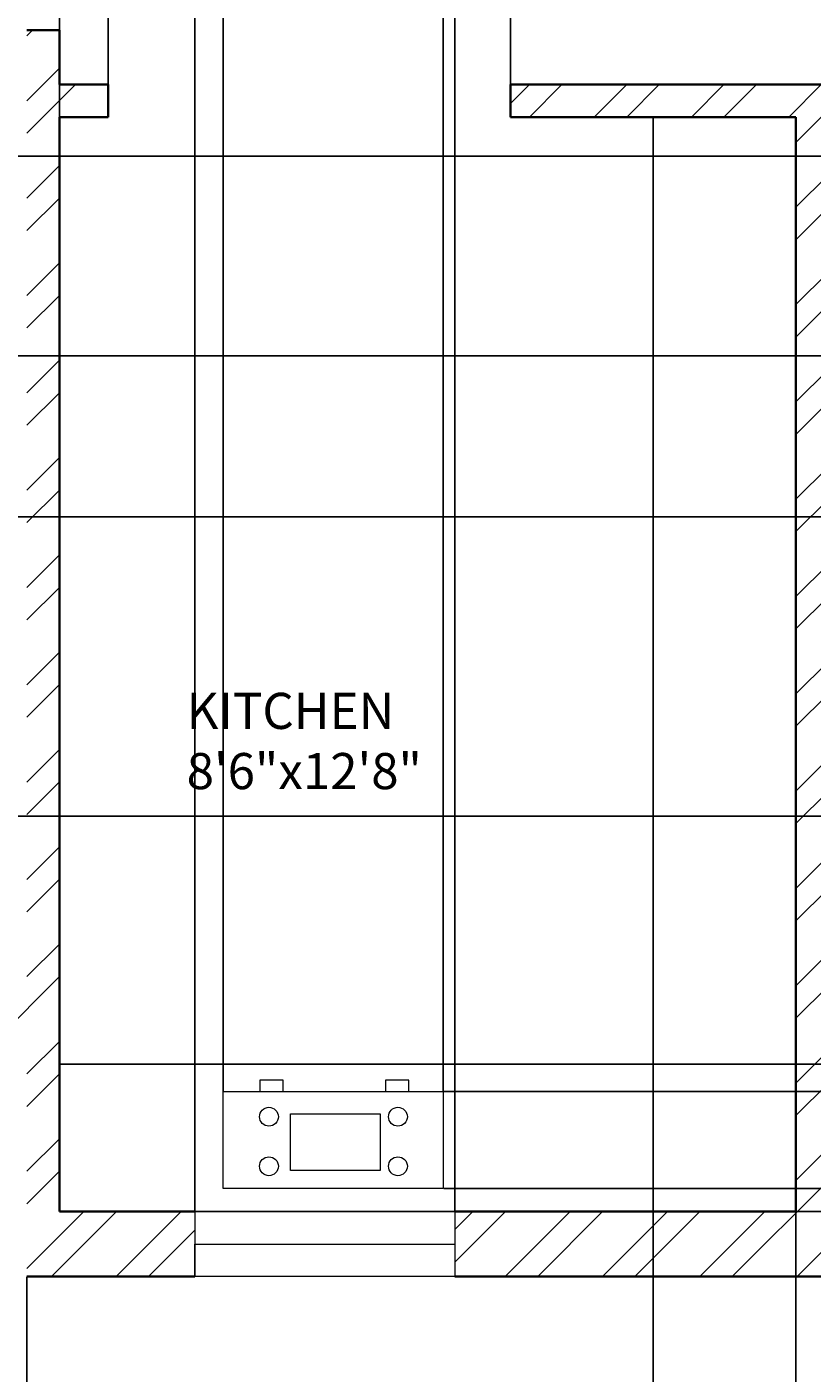
# Model space of a CAD drawing. Units: inches. Extents: x 2529 to 3014, y 1203 to 2262.
# Tile 5 of 13: x 2733 to 2842, y 1560 to 1746. Entities that reach past the tile are written whole.
import ezdxf

# ---------------------------------------------------------------- set-up
doc = ezdxf.new("R2010")
doc.units = ezdxf.units.IN
for name, color, linetype, lineweight in [('A-ANNO-DIMS', 2, 'Continuous', 18), ('A-AREA-IDEN', 7, 'Continuous', 18), ('A-EQPM', 8, 'Continuous', 18), ('A-FLOR-CASE', 7, 'Continuous', 25), ('A-GLAZ', 191, 'Continuous', 18), ('A-WALL', 7, 'Continuous', 35), ('A-WALL-PATT', 143, 'Continuous', 13)]:
    doc.layers.add(name, color=color, linetype=linetype, lineweight=lineweight)
doc.styles.get("Standard").update_dxf_attribs({"font": 'arial.ttf'})
doc.dimstyles.get("Standard").update_dxf_attribs({"dimtxt": 0.18, "dimasz": 0.18, "dimexe": 0.18, "dimexo": 0.0625, "dimgap": 0.09, "dimtad": 0, "dimtih": 1, "dimtoh": 1, "dimdec": 4, "dimzin": 0, "dimdsep": 46, "dimtxsty": 'Standard', "dimcen": 0.09, "dimadec": 0, "dimazin": 0, "dimtfac": 1, "dimtdec": 4, "dimtofl": 0, "dimtmove": 0, "dimatfit": 3, "dimfxl": 1, "dimtolj": 1, "dimtzin": 0, "dimarcsym": 0})

# ---------------------------------------------------------------- blocks, each defined once
blk = doc.blocks.new('*D19')
at = {"layer": 'A-ANNO-DIMS', "color": 0, "lineweight": -2, "transparency": 16777216}
for p, q in [((2839.56, 1582.44), (2839.56, 1483.77)), ((2733.06, 1573.44), (2733.06, 1483.77)), ((2733.24, 1483.95), (2785.92, 1483.95)), ((2839.38, 1483.95), (2786.69, 1483.95))]:
    blk.add_line(p, q, dxfattribs=at)
at = {"layer": 'A-ANNO-DIMS', "color": 0, "transparency": 16777216}
for points in [[(2733.24, 1483.98), (2733.24, 1483.92), (2733.06, 1483.95)], [(2839.38, 1483.98), (2839.38, 1483.92), (2839.56, 1483.95)]]:
    blk.add_solid(points, dxfattribs=at)
at = {"layer": 'Defpoints', "color": 0, "transparency": 16777216}
for p in [(2839.56, 1582.5), (2733.06, 1573.5), (2839.56, 1483.95)]:
    blk.add_point(p, dxfattribs=at)
at = {"layer": 'A-ANNO-DIMS', "color": 0, "transparency": 16777216, "insert": (2786.31, 1483.95), "char_height": 0.18, "attachment_point": 5}
blk.add_mtext('\\A1;106.5', dxfattribs=at)
blk = doc.blocks.new('*D20')
at = {"layer": 'A-ANNO-DIMS', "color": 0, "lineweight": -2, "transparency": 16777216}
for p, q in [((2839.56, 1582.44), (2839.56, 1483.77)), ((2972.06, 1573.44), (2972.06, 1483.77)), ((2839.74, 1483.95), (2905.42, 1483.95)), ((2971.88, 1483.95), (2906.19, 1483.95))]:
    blk.add_line(p, q, dxfattribs=at)
at = {"layer": 'A-ANNO-DIMS', "color": 0, "transparency": 16777216}
for points in [[(2839.74, 1483.98), (2839.74, 1483.92), (2839.56, 1483.95)], [(2971.88, 1483.98), (2971.88, 1483.92), (2972.06, 1483.95)]]:
    blk.add_solid(points, dxfattribs=at)
at = {"layer": 'Defpoints', "color": 0, "transparency": 16777216}
for p in [(2839.56, 1582.5), (2972.06, 1573.5), (2972.06, 1483.95)]:
    blk.add_point(p, dxfattribs=at)
at = {"layer": 'A-ANNO-DIMS', "color": 0, "transparency": 16777216, "insert": (2905.81, 1483.95), "char_height": 0.18, "attachment_point": 5}
blk.add_mtext('\\A1;132.5', dxfattribs=at)
blk = doc.blocks.new('*D36')
at = {"layer": 'A-ANNO-DIMS', "color": 0, "lineweight": -2, "transparency": 16777216}
for p, q in [((2737.56, 1582.57), (2737.56, 2243.11)), ((2737.74, 2242.93), (2746.49, 2242.93)), ((2756.15, 2242.93), (2747.4, 2242.93)), ((2756.33, 1582.57), (2756.33, 2243.11))]:
    blk.add_line(p, q, dxfattribs=at)
at = {"layer": 'A-ANNO-DIMS', "color": 0, "transparency": 16777216}
for points in [[(2737.74, 2242.96), (2737.74, 2242.9), (2737.56, 2242.93)], [(2756.15, 2242.96), (2756.15, 2242.9), (2756.33, 2242.93)]]:
    blk.add_solid(points, dxfattribs=at)
at = {"layer": 'Defpoints', "color": 0, "transparency": 16777216}
for p in [(2756.33, 2242.93), (2737.56, 1582.5), (2756.33, 1582.5)]:
    blk.add_point(p, dxfattribs=at)
at = {"layer": 'A-ANNO-DIMS', "color": 0, "transparency": 16777216, "insert": (2746.94, 2242.93), "char_height": 0.18, "attachment_point": 5}
blk.add_mtext('\\A1;18.778', dxfattribs=at)
blk = doc.blocks.new('*D37')
at = {"layer": 'A-ANNO-DIMS', "color": 0, "lineweight": -2, "transparency": 16777216}
for p, q in [((2756.33, 1582.57), (2756.33, 2243.11)), ((2756.51, 2242.93), (2774.11, 2242.93)), ((2792.15, 2242.93), (2774.55, 2242.93)), ((2792.33, 1582.57), (2792.33, 2243.11))]:
    blk.add_line(p, q, dxfattribs=at)
at = {"layer": 'A-ANNO-DIMS', "color": 0, "transparency": 16777216}
for points in [[(2756.51, 2242.96), (2756.51, 2242.9), (2756.33, 2242.93)], [(2792.15, 2242.96), (2792.15, 2242.9), (2792.33, 2242.93)]]:
    blk.add_solid(points, dxfattribs=at)
at = {"layer": 'Defpoints', "color": 0, "transparency": 16777216}
for p in [(2792.33, 2242.93), (2756.33, 1582.5), (2792.33, 1582.5)]:
    blk.add_point(p, dxfattribs=at)
at = {"layer": 'A-ANNO-DIMS', "color": 0, "transparency": 16777216, "insert": (2774.33, 2242.93), "char_height": 0.18, "attachment_point": 5}
blk.add_mtext('\\A1;36', dxfattribs=at)
blk = doc.blocks.new('*D40')
at = {"layer": 'A-ANNO-DIMS', "color": 0, "lineweight": -2, "transparency": 16777216}
for p, q in [((2744.32, 1738.57), (2744.32, 2243.11)), ((2744.5, 2242.93), (2771.84, 2242.93)), ((2799.84, 2242.93), (2772.49, 2242.93)), ((2800.02, 1738.57), (2800.02, 2243.11))]:
    blk.add_line(p, q, dxfattribs=at)
at = {"layer": 'A-ANNO-DIMS', "color": 0, "transparency": 16777216}
for points in [[(2744.5, 2242.96), (2744.5, 2242.9), (2744.32, 2242.93)], [(2799.84, 2242.96), (2799.84, 2242.9), (2800.02, 2242.93)]]:
    blk.add_solid(points, dxfattribs=at)
at = {"layer": 'Defpoints', "color": 0, "transparency": 16777216}
for p in [(2800.02, 2242.93), (2744.32, 1738.5), (2800.02, 1738.5)]:
    blk.add_point(p, dxfattribs=at)
at = {"layer": 'A-ANNO-DIMS', "color": 0, "transparency": 16777216, "insert": (2772.17, 2242.93), "char_height": 0.18, "attachment_point": 5}
blk.add_mtext('\\A1;55.7', dxfattribs=at)
blk = doc.blocks.new('*D41')
at = {"layer": 'A-ANNO-DIMS', "color": 0, "lineweight": -2, "transparency": 16777216}
for p, q in [((2819.79, 1733.94), (2819.79, 1483.77)), ((2839.56, 1733.94), (2839.56, 1483.77)), ((2819.97, 1483.95), (2829.29, 1483.95)), ((2839.38, 1483.95), (2830.06, 1483.95))]:
    blk.add_line(p, q, dxfattribs=at)
at = {"layer": 'A-ANNO-DIMS', "color": 0, "transparency": 16777216}
for points in [[(2819.97, 1483.98), (2819.97, 1483.92), (2819.79, 1483.95)], [(2839.38, 1483.98), (2839.38, 1483.92), (2839.56, 1483.95)]]:
    blk.add_solid(points, dxfattribs=at)
at = {"layer": 'Defpoints', "color": 0, "transparency": 16777216}
for p in [(2819.79, 1734), (2839.56, 1734), (2819.79, 1483.95)]:
    blk.add_point(p, dxfattribs=at)
at = {"layer": 'A-ANNO-DIMS', "color": 0, "transparency": 16777216, "insert": (2829.67, 1483.95), "char_height": 0.18, "attachment_point": 5}
blk.add_mtext('\\A1;19.77', dxfattribs=at)
blk = doc.blocks.new('*D43')
at = {"layer": 'A-ANNO-DIMS', "color": 0, "lineweight": -2, "transparency": 16777216}
for p, q in [((2616.77, 1700.93), (3007.66, 1700.93)), ((3007.48, 1700.75), (3007.48, 1669.26)), ((3007.48, 1637.41), (3007.48, 1668.9)), ((2616.77, 1637.23), (3007.66, 1637.23))]:
    blk.add_line(p, q, dxfattribs=at)
at = {"layer": 'A-ANNO-DIMS', "color": 0, "transparency": 16777216}
for points in [[(3007.45, 1700.75), (3007.51, 1700.75), (3007.48, 1700.93)], [(3007.45, 1637.41), (3007.51, 1637.41), (3007.48, 1637.23)]]:
    blk.add_solid(points, dxfattribs=at)
at = {"layer": 'Defpoints', "color": 0, "transparency": 16777216}
for p in [(2616.71, 1700.93), (3007.48, 1700.93), (2616.71, 1637.23)]:
    blk.add_point(p, dxfattribs=at)
at = {"layer": 'A-ANNO-DIMS', "color": 0, "transparency": 16777216, "insert": (3007.48, 1669.08), "char_height": 0.18, "attachment_point": 5}
blk.add_mtext('\\A1;63.7', dxfattribs=at)
blk = doc.blocks.new('*D45')
at = {"layer": 'A-ANNO-DIMS', "color": 0, "lineweight": -2, "transparency": 16777216}
for p, q in [((2655.95, 1728.6), (3007.66, 1728.6)), ((3007.48, 1728.42), (3007.48, 1703.82)), ((3007.48, 1678.86), (3007.48, 1703.46)), ((2655.95, 1678.68), (3007.66, 1678.68))]:
    blk.add_line(p, q, dxfattribs=at)
at = {"layer": 'A-ANNO-DIMS', "color": 0, "transparency": 16777216}
for points in [[(3007.45, 1728.42), (3007.51, 1728.42), (3007.48, 1728.6)], [(3007.45, 1678.86), (3007.51, 1678.86), (3007.48, 1678.68)]]:
    blk.add_solid(points, dxfattribs=at)
at = {"layer": 'Defpoints', "color": 0, "transparency": 16777216}
for p in [(2655.89, 1728.6), (3007.48, 1728.6), (2655.89, 1678.68)]:
    blk.add_point(p, dxfattribs=at)
at = {"layer": 'A-ANNO-DIMS', "color": 0, "transparency": 16777216, "insert": (3007.48, 1703.64), "char_height": 0.18, "attachment_point": 5}
blk.add_mtext('\\A1;49.92', dxfattribs=at)
blk = doc.blocks.new('*D78')
at = {"layer": 'A-ANNO-DIMS', "color": 0, "lineweight": -2, "transparency": 16777216}
for p, q in [((2760.22, 1599.16), (2760.22, 2243.11)), ((2760.4, 2242.93), (2775.15, 2242.93)), ((2790.54, 2242.93), (2775.8, 2242.93)), ((2790.72, 1599.16), (2790.72, 2243.11))]:
    blk.add_line(p, q, dxfattribs=at)
at = {"layer": 'A-ANNO-DIMS', "color": 0, "transparency": 16777216}
for points in [[(2760.4, 2242.96), (2760.4, 2242.9), (2760.22, 2242.93)], [(2790.54, 2242.96), (2790.54, 2242.9), (2790.72, 2242.93)]]:
    blk.add_solid(points, dxfattribs=at)
at = {"layer": 'Defpoints', "color": 0, "transparency": 16777216}
for p in [(2790.72, 2242.93), (2760.22, 1599.1), (2790.72, 1599.1)]:
    blk.add_point(p, dxfattribs=at)
at = {"layer": 'A-ANNO-DIMS', "color": 0, "transparency": 16777216, "insert": (2775.47, 2242.93), "char_height": 0.18, "attachment_point": 5}
blk.add_mtext('\\A1;30.5', dxfattribs=at)
blk = doc.blocks.new('*D79')
at = {"layer": 'A-ANNO-DIMS', "color": 0, "lineweight": -2, "transparency": 16777216}
for p, q in [((2790.78, 1599.1), (3007.66, 1599.1)), ((3007.48, 1598.92), (3007.48, 1592.58)), ((3007.48, 1585.88), (3007.48, 1592.22)), ((2790.78, 1585.7), (3007.66, 1585.7))]:
    blk.add_line(p, q, dxfattribs=at)
at = {"layer": 'A-ANNO-DIMS', "color": 0, "transparency": 16777216}
for points in [[(3007.45, 1598.92), (3007.51, 1598.92), (3007.48, 1599.1)], [(3007.45, 1585.88), (3007.51, 1585.88), (3007.48, 1585.7)]]:
    blk.add_solid(points, dxfattribs=at)
at = {"layer": 'Defpoints', "color": 0, "transparency": 16777216}
for p in [(2790.72, 1599.1), (3007.48, 1599.1), (2790.72, 1585.7)]:
    blk.add_point(p, dxfattribs=at)
at = {"layer": 'A-ANNO-DIMS', "color": 0, "transparency": 16777216, "insert": (3007.48, 1592.4), "char_height": 0.18, "attachment_point": 5}
blk.add_mtext('\\A1;13.397', dxfattribs=at)
blk = doc.blocks.new('*D80')
at = {"layer": 'A-ANNO-DIMS', "color": 0, "lineweight": -2, "transparency": 16777216}
for p, q in [((2737.62, 1602.91), (3007.66, 1602.91)), ((3007.48, 1602.73), (3007.48, 1592.89)), ((3007.48, 1582.68), (3007.48, 1592.52)), ((2737.62, 1582.5), (3007.66, 1582.5))]:
    blk.add_line(p, q, dxfattribs=at)
at = {"layer": 'A-ANNO-DIMS', "color": 0, "transparency": 16777216}
for points in [[(3007.45, 1602.73), (3007.51, 1602.73), (3007.48, 1602.91)], [(3007.45, 1582.68), (3007.51, 1582.68), (3007.48, 1582.5)]]:
    blk.add_solid(points, dxfattribs=at)
at = {"layer": 'Defpoints', "color": 0, "transparency": 16777216}
for p in [(2737.56, 1602.91), (3007.48, 1602.91), (2737.56, 1582.5)]:
    blk.add_point(p, dxfattribs=at)
at = {"layer": 'A-ANNO-DIMS', "color": 0, "transparency": 16777216, "insert": (3007.48, 1592.71), "char_height": 0.18, "attachment_point": 5}
blk.add_mtext('\\A1;20.406', dxfattribs=at)

msp = doc.modelspace()

# ---------------------------------------------------------------- hatches: boundary and pattern name
at = {"layer": 'A-WALL-PATT'}
h = msp.add_hatch(dxfattribs=at)
h.set_pattern_fill('ANSI32', color=256)
h.paths.add_polyline_path([(2686.5554, 2106.5032), (2622.0554, 2106.5032), (2622.0554, 2109.2964), (2617.4223, 2109.2964), (2613.0554, 2109.2964), (2613.0554, 2106.5032), (2577.0554, 2106.5032), (2577.0554, 2092.6918), (2586.0554, 2092.6918), (2586.0554, 2102.0032), (2682.0554, 2102.0032), (2682.0554, 2099.9833), (2686.5554, 2099.9833), (2686.5554, 2102.0032)])
h.paths.add_polyline_path([(2695.2249, 2054.0032), (2686.5554, 2054.0032), (2686.5554, 2080.2316), (2684.3054, 2080.2316), (2682.0554, 2080.2316), (2682.0554, 2054.0032), (2586.0554, 2054.0032), (2586.0554, 2068.6918), (2577.0554, 2068.6918), (2577.0554, 2019.1229), (2586.0554, 2019.1229), (2586.0554, 2049.5032), (2695.2249, 2049.5032)])
h.paths.add_polyline_path([(2737.5554, 2049.5032), (2866.5554, 2049.5032), (2866.5554, 2045.0233), (2871.0554, 2045.0233), (2871.0554, 2049.5032), (2871.0554, 2172.5032), (2866.5554, 2172.5032), (2829.1265, 2172.5032), (2829.1265, 2168.0032), (2866.5554, 2168.0032), (2866.5554, 2054.0032), (2737.5554, 2054.0032), (2737.5554, 2056.4892), (2735.3054, 2056.4892), (2733.0554, 2056.4892), (2733.0554, 2049.5032), (2733.0554, 1917.5032), (2733.0554, 1913.0032), (2871.0554, 1913.0032), (2871.0554, 1924.9149), (2868.8054, 1924.9149), (2866.5554, 1924.9149), (2866.5554, 1917.5032), (2737.5554, 1917.5032)], flags=17)
h.paths.add_polyline_path([(2972.0554, 2207.5032), (2613.0554, 2207.5032), (2613.0554, 2205.5032), (2613.0554, 2188.9366), (2622.0554, 2188.9366), (2622.0554, 2198.5032), (2733.0554, 2198.5032), (2733.0554, 2084.8053), (2735.3054, 2084.8053), (2737.5554, 2084.8053), (2737.5554, 2168.0032), (2769.1265, 2168.0032), (2769.1265, 2170.2532), (2769.1265, 2172.5032), (2737.5554, 2172.5032), (2737.5554, 2198.5032), (2963.0554, 2198.5032), (2963.0554, 2093.5032), (2912.0586, 2093.5032), (2912.0586, 2089.0032), (2918.5554, 2089.0032), (2918.5554, 2031.8749), (2923.0554, 2031.8749), (2923.0554, 2089.0032), (2963.0554, 2089.0032), (2963.0554, 2010.0032), (2923.0554, 2010.0032), (2923.0554, 2011.9417), (2918.5554, 2011.9417), (2918.5554, 2003.1338), (2923.0554, 2003.1338), (2923.0554, 2005.5032), (2963.0554, 2005.5032), (2963.0554, 1917.5032), (2963.0554, 1691.0776), (2972.0554, 1691.0776), (2972.0554, 1917.5032)])
h.paths.add_polyline_path([(2963.0554, 1945.5032), (2923.0554, 1945.5032), (2923.0554, 1983.0571), (2920.8054, 1983.0571), (2918.5554, 1983.0571), (2918.5554, 1941.0032), (2963.0554, 1941.0032)], flags=17)
h.paths.add_polyline_path([(2930.3679, 1788.7532), (2930.3679, 1791.0032), (2894.8637, 1791.0032), (2894.8637, 1786.5032), (2900.5554, 1786.5032), (2900.5554, 1784.6931), (2905.0554, 1784.6931), (2905.0554, 1786.5032), (2930.3679, 1786.5032)], flags=17)
h.paths.add_polyline_path([(2963.0554, 1791.0032), (2954.3679, 1791.0032), (2954.3679, 1786.5032), (2963.0554, 1786.5032)], flags=17)
h.paths.add_polyline_path([(2871.0554, 1853.0032), (2919.0554, 1853.0032), (2919.0554, 1847.0972), (2923.5554, 1847.0972), (2923.5554, 1853.0032), (2923.5554, 1857.5032), (2871.0554, 1857.5032), (2871.0554, 1871.7024), (2866.5554, 1871.7024), (2866.5554, 1791.0032), (2737.5554, 1791.0032), (2737.5554, 1806.6712), (2735.3054, 1806.6712), (2733.0554, 1806.6712), (2733.0554, 1791.0032), (2733.0554, 1786.5032), (2733.0554, 1780.6235), (2737.5554, 1780.6235), (2737.5554, 1786.5032), (2872.8745, 1786.5032), (2872.8745, 1788.7532), (2872.8745, 1791.0032), (2871.0554, 1791.0032)], flags=17)
h.paths.add_polyline_path([(2844.0554, 1734.0032), (2848.2652, 1734.0032), (2848.2652, 1738.5032), (2800.0167, 1738.5032), (2800.0167, 1734.0032), (2839.5554, 1734.0032), (2839.5554, 1582.5032), (2792.3334, 1582.5032), (2792.3334, 1573.5032), (2871.4433, 1573.5032), (2871.4433, 1578.0032), (2871.4433, 1582.5032), (2844.0554, 1582.5032)])
h.paths.add_polyline_path([(2972.0554, 1631.0776), (2963.0554, 1631.0776), (2963.0554, 1582.5032), (2931.4433, 1582.5032), (2931.4433, 1573.5032), (2972.0554, 1573.5032)])
h.paths.add_polyline_path([(2756.3334, 1582.5032), (2737.5554, 1582.5032), (2737.5554, 1734.0032), (2744.3201, 1734.0032), (2744.3201, 1738.5032), (2737.5554, 1738.5032), (2737.5554, 1746.0094), (2733.0554, 1746.0094), (2733.0554, 1738.5032), (2733.0554, 1612.5032), (2728.2475, 1612.5032), (2728.2475, 1603.5032), (2733.0554, 1603.5032), (2733.0554, 1582.5032), (2733.0554, 1573.5032), (2756.3334, 1573.5032), (2756.3334, 1578.0032)])
h.paths.add_polyline_path([(2695.7662, 1612.5032), (2658.4771, 1612.5032), (2658.4771, 1603.5032), (2695.7662, 1603.5032), (2695.7662, 1608.0032)])
h.paths.add_polyline_path([(2586.0554, 1686.9483), (2577.0554, 1686.9483), (2577.0554, 1603.5032), (2598.4771, 1603.5032), (2598.4771, 1608.0032), (2598.4771, 1612.5032), (2586.0554, 1612.5032)])
h.paths.add_polyline_path([(2683.2727, 1791.0032), (2586.0554, 1791.0032), (2586.0554, 1815.6736), (2581.5554, 1815.6736), (2577.0554, 1815.6736), (2577.0554, 1746.9483), (2586.0554, 1746.9483), (2586.0554, 1786.5032), (2683.2727, 1786.5032)])
h.paths.add_polyline_path([(2586.0554, 1959.1229), (2577.0554, 1959.1229), (2577.0554, 1875.6736), (2586.0554, 1875.6736), (2586.0554, 1913.0032), (2683.2727, 1913.0032), (2683.2727, 1917.5032), (2586.0554, 1917.5032)])

# ---------------------------------------------------------------- linework, layer by layer
at = {"layer": 'A-EQPM'}
for points in [[(2765.311, 1599.0994), (2768.5415, 1599.0994), (2768.5415, 1600.6937), (2765.311, 1600.6937)], [(2782.7381, 1599.0994), (2785.9686, 1599.0994), (2785.9686, 1600.6937), (2782.7381, 1600.6937)], [(2760.2227, 1599.0994), (2790.721, 1599.0994), (2790.721, 1585.702), (2760.2227, 1585.702)], [(2769.5469, 1596.0204), (2781.9822, 1596.0204), (2781.9822, 1588.1929), (2769.5469, 1588.1929)]]:
    msp.add_lwpolyline(points, close=True, dxfattribs=at)
for centre in [(2766.5826, 1595.629), (2784.4431, 1595.629), (2766.5826, 1588.7706), (2784.4431, 1588.7706)]:
    msp.add_circle(centre, 1.3046, dxfattribs=at)
at = {"layer": 'A-FLOR-CASE'}
for p, q in [((2819.786, 1734.0032), (2819.786, 1602.9088)), ((2819.786, 1602.9088), (2737.5554, 1602.9088))]:
    msp.add_line(p, q, dxfattribs=at)
at = {"layer": 'A-GLAZ'}
for p, q in [((2756.3334, 1582.5032), (2756.3334, 1573.5032)), ((2756.3334, 1582.5032), (2792.3334, 1582.5032)), ((2792.3334, 1582.5032), (2792.3334, 1573.5032)), ((2756.3334, 1573.5032), (2756.3334, 1578.0032)), ((2756.3334, 1578.0032), (2792.3334, 1578.0032)), ((2792.3334, 1573.5032), (2756.3334, 1573.5032))]:
    msp.add_line(p, q, dxfattribs=at)
at = {"layer": 'A-WALL'}
for p, q in [((2733.0554, 1746.0094), (2737.5554, 1746.0094)), ((2737.5554, 1746.0094), (2737.5554, 1738.5032)), ((2737.5554, 1738.5032), (2744.3201, 1738.5032)), ((2744.3201, 1738.5032), (2744.3201, 1734.0032)), ((2800.0167, 1738.5032), (2800.0167, 1734.0032)), ((2800.0167, 1738.5032), (2848.2652, 1738.5032)), ((2737.5554, 1734.0032), (2737.5554, 1582.5032)), ((2737.5554, 1734.0032), (2744.3201, 1734.0032)), ((2737.5554, 1734.0032), (2744.3201, 1734.0032)), ((2800.0167, 1734.0032), (2839.5554, 1734.0032)), ((2800.0167, 1734.0032), (2839.5554, 1734.0032)), ((2839.5554, 1734.0032), (2839.5554, 1582.5032)), ((2756.3334, 1582.5032), (2737.5554, 1582.5032)), ((2839.5554, 1582.5032), (2792.3334, 1582.5032)), ((2756.3334, 1573.5032), (2733.0554, 1573.5032)), ((2871.4433, 1573.5032), (2792.3334, 1573.5032))]:
    msp.add_line(p, q, dxfattribs=at)

# ---------------------------------------------------------------- texts
at = {"layer": 'A-AREA-IDEN', "insert": (2755.1769, 1654.3055), "char_height": 5, "attachment_point": 1}
msp.add_mtext_dynamic_manual_height_columns('KITCHEN\\P8\'6"x12\'8"', width=113.409094, gutter_width=12.5, heights=[0], dxfattribs=at)

# ---------------------------------------------------------------- dimensions: what is measured, and where the dimension line sits
at = {"layer": 'A-ANNO-DIMS'}
for base, p1, p2, override, picture, middle in [((2756.3334, 2242.9282), (2737.5554, 1582.5032), (2756.3334, 1582.5032), {"dimdec": 3, "dimlfac": 1, "dimrnd": 0, "dimzin": 0, "dimdsep": 46, "dimlunit": 2}, '*D36', (2746.9444, 2242.9282)), ((2800.0167, 2242.9282), (2744.3201, 1738.5032), (2800.0167, 1738.5032), {"dimdec": 1, "dimlfac": 1, "dimrnd": 0, "dimzin": 0, "dimdsep": 46, "dimlunit": 2}, '*D40', (2772.1684, 2242.9282)), ((2792.3334, 2242.9282), (2756.3334, 1582.5032), (2792.3334, 1582.5032), {"dimdec": 0, "dimlfac": 1, "dimrnd": 0, "dimzin": 0, "dimdsep": 46, "dimlunit": 2}, '*D37', (2774.3334, 2242.9282)), ((2790.721, 2242.9282), (2760.2227, 1599.0994), (2790.721, 1599.0994), {"dimdec": 1, "dimlfac": 1, "dimrnd": 0, "dimzin": 0, "dimdsep": 46, "dimlunit": 2}, '*D78', (2775.4718, 2242.9282)), ((2819.786, 1483.9492), (2839.5554, 1734.0032), (2819.786, 1734.0032), {"dimdec": 2, "dimlfac": 1, "dimrnd": 0, "dimzin": 0, "dimdsep": 46, "dimlunit": 2}, '*D41', (2829.6707, 1483.9492)), ((2839.5554, 1483.9492), (2733.0554, 1573.5032), (2839.5554, 1582.5032), {"dimdec": 1, "dimlfac": 1, "dimrnd": 0, "dimzin": 0, "dimdsep": 46, "dimlunit": 2}, '*D19', (2786.3054, 1483.9492)), ((2972.0554, 1483.9492), (2839.5554, 1582.5032), (2972.0554, 1573.5032), {"dimdec": 1, "dimlfac": 1, "dimrnd": 0, "dimzin": 0, "dimdsep": 46, "dimlunit": 2}, '*D20', (2905.8054, 1483.9492))]:
    dim = msp.add_linear_dim(base=base, p1=p1, p2=p2, dimstyle='Standard', override=override, dxfattribs=at)
    dim.commit()
    dim.dimension.update_dxf_attribs({"geometry": picture, "text_midpoint": middle})
for base, p1, p2, override, picture, middle in [((3007.4804, 1728.5992), (2655.8904, 1678.6815), (2655.8904, 1728.5992), {"dimdec": 2, "dimlfac": 1, "dimrnd": 0, "dimzin": 0, "dimdsep": 46, "dimlunit": 2}, '*D45', (3007.4804, 1703.6403)), ((3007.4804, 1700.9333), (2616.7105, 1637.2315), (2616.7105, 1700.9333), {"dimdec": 1, "dimlfac": 1, "dimrnd": 0, "dimzin": 0, "dimdsep": 46, "dimlunit": 2}, '*D43', (3007.4804, 1669.0824)), ((3007.4804, 1602.9088), (2737.5554, 1582.5032), (2737.5554, 1602.9088), {"dimdec": 3, "dimlfac": 1, "dimrnd": 0, "dimzin": 0, "dimdsep": 46, "dimlunit": 2}, '*D80', (3007.4804, 1592.706)), ((3007.4804, 1599.0994), (2790.721, 1585.702), (2790.721, 1599.0994), {"dimdec": 3, "dimlfac": 1, "dimrnd": 0, "dimzin": 0, "dimdsep": 46, "dimlunit": 2}, '*D79', (3007.4804, 1592.4007))]:
    dim = msp.add_linear_dim(base=base, p1=p1, p2=p2, angle=90, dimstyle='Standard', override=override, dxfattribs=at)
    dim.commit()
    dim.dimension.update_dxf_attribs({"geometry": picture, "text_midpoint": middle})

doc.saveas('drawing.dxf')
